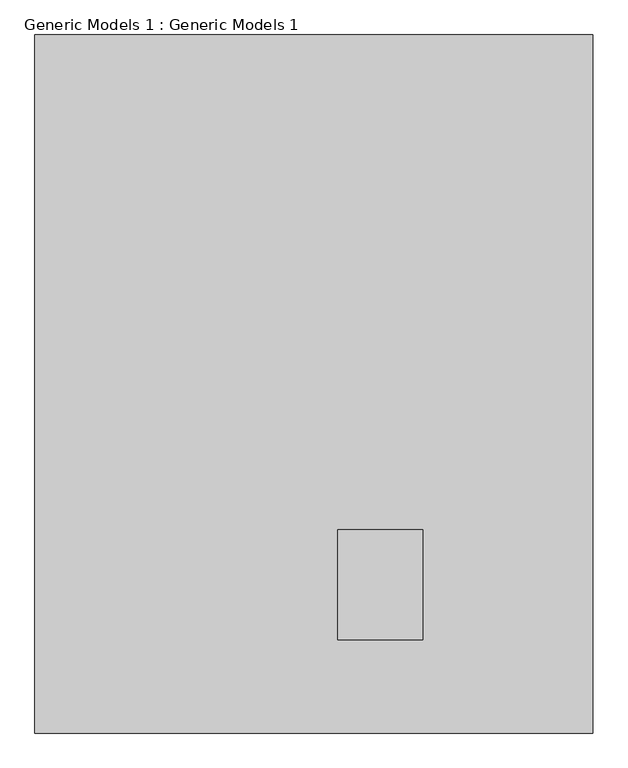
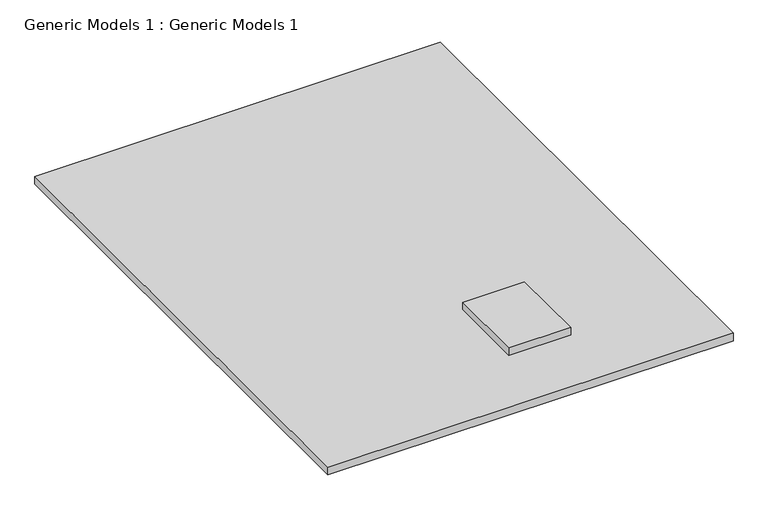
"""IFC4 building model written with IfcOpenShell, lengths in millimetres: proxy geometry, Generic Models 1 : Generic Models 1."""

from ifc_helpers import new_model, si_unit, frame, origin, origin_with_axes, place, context, project, spatial, polyline, outline, extrude, source, transform, mapped, element, save


def generic_models_1_generic_models_1_f3807b65(model_context):
    return source(origin(), model_context, "Body", "SweptSolid", [
        extrude(outline(polyline([(-4816.0838989, 3786.0597869), (-4816.0838989, -15574.9202535), (-20282.6509421, -15574.9202535), (-20282.6509421, 3786.0597869), (-4816.0838989, 3786.0597869)])), frame((0.0, 0.0, -304.8), z_axis=(0.0, 0.0, 1.0), x_axis=(1.0, 0.0, 0.0)), (0.0, 0.0, 1.0), 304.8),
        extrude(outline(polyline([(-9523.0624893, -9939.2040375), (-9523.0624893, -12987.2040375), (-11885.2624893, -12987.2040375), (-11885.2624893, -9939.2040375), (-9523.0624893, -9939.2040375)])), origin_with_axes(), (0.0, 0.0, 1.0), 304.8),
    ])


if __name__ == "__main__":
    model = new_model("IFC4")
    model_context = context("Model", 3, world=origin())
    ifc_project = project(units=[si_unit("LENGTHUNIT", "METRE", prefix="MILLI")], contexts=[model_context])
    site = spatial("IfcSite", under=ifc_project)
    building = spatial("IfcBuilding", under=site)
    placement = place(None, origin())
    generic_models_1_generic_models_1_shape = generic_models_1_generic_models_1_f3807b65(model_context)
    element("IfcBuildingElementProxy", 1, Name="Generic Models 1 : Generic Models 1", ObjectType="Generic Models 1 : Generic Models 1", at=placement, inside=building, context=model_context, shape_type="MappedRepresentation", body=[
        mapped(generic_models_1_generic_models_1_shape, transform((0.0, 0.0, 0.0), x_axis=(1.0, 0.0, 0.0), y_axis=(0.0, 1.0, 0.0), z_axis=(0.0, 0.0, 1.0))),
    ])
    save(model, "model.ifc")
